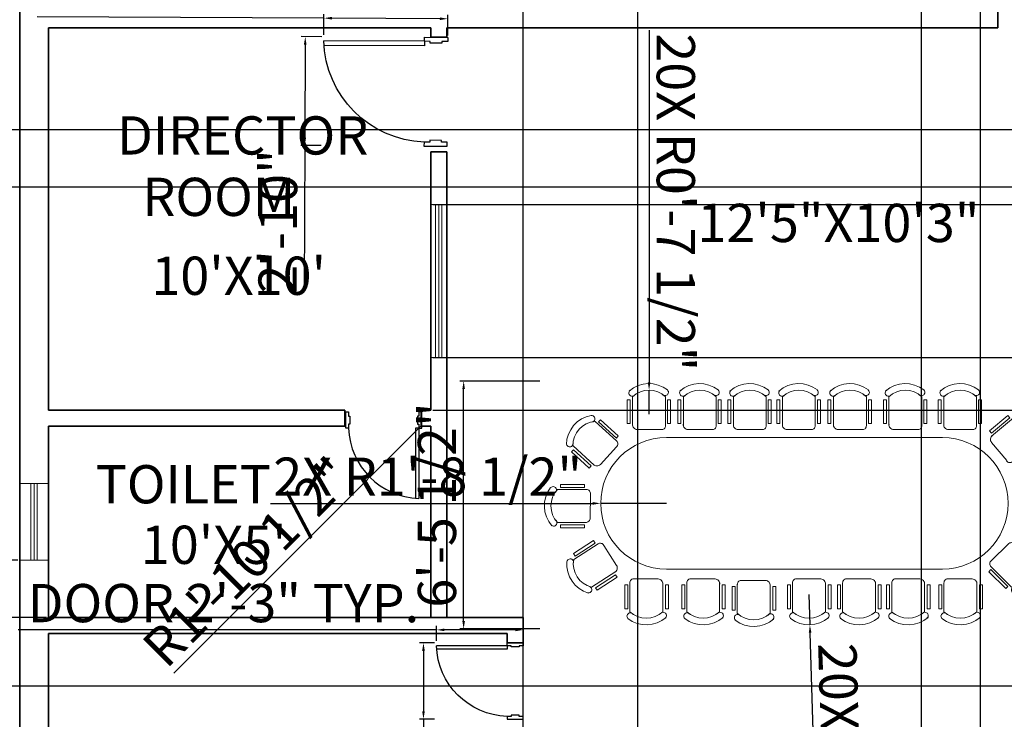
# Model space of a CAD drawing. Units: inches. Extents: x 2319 to 3765, y 2872 to 3950.
# Tile 3 of 9: x 2474 to 2783, y 3087 to 3306. Entities that reach past the tile are written whole.
import ezdxf

# ---------------------------------------------------------------- set-up
doc = ezdxf.new("R2010")
doc.units = ezdxf.units.IN
for name, color, linetype, lineweight in [('A-ANNO-DIMS', 2, 'Continuous', 18), ('A-ANNO-SYMB', 3, 'Continuous', 25), ('A-AREA-IDEN', 7, 'Continuous', 18), ('A-DOOR', 3, 'Continuous', 25), ('A-FURN', 8, 'Continuous', 18), ('A-GLAZ', 4, 'Continuous', 18), ('A-WALL', 7, 'Continuous', 35)]:
    doc.layers.add(name, color=color, linetype=linetype, lineweight=lineweight)
doc.styles.get("Standard").update_dxf_attribs({"font": 'arial.ttf'})
doc.dimstyles.new('ISO-25', dxfattribs={"dimtxt": 12, "dimasz": 2.5, "dimexe": 1.25, "dimexo": 0.625, "dimtad": 1, "dimdec": 0, "dimlunit": 3, "dimtxsty": 'Standard', "dimcen": 2.5, "dimadec": 0, "dimazin": 0, "dimtfac": 1, "dimtdec": 0, "dimtmove": 0, "dimatfit": 3, "dimfxl": 1, "dimarcsym": 0})

# ---------------------------------------------------------------- blocks, each defined once
blk = doc.blocks.new('A$C769D55ED')
for p, q in [((33.6, 192), (33.6, 1024.8)), ((72, 192), (72, 1023.9)), ((0, 192), (0, 0)), ((33.6, 192), (0, 192)), ((33.6, 144), (33.6, 192)), ((48, 144), (33.6, 144)), ((48, 48), (48, 144)), ((33.6, 0), (33.6, 48)), ((33.6, 48), (48, 48)), ((0, 0), (33.6, 0))]:
    blk.add_line(p, q)
blk.add_lwpolyline([(33.6, 192), (72, 192)])
blk.add_lwpolyline([(900, 192), (900, 0), (866.4, 0), (866.4, 48), (852, 48), (852, 144), (866.4, 144), (866.4, 192)], close=True)
blk.add_arc((7.2, 165.6), 859.6, 1.76235, 88.23765)
blk = doc.blocks.new('A$C0EDB4AB9')
at = {"linetype": 'ByBlock'}
for p, q in [((1257, 3447), (1257, 3084)), ((1303, 3447), (1257, 3447)), ((1303, 3084), (1303, 3447)), ((1342, 3055), (1342, 3493)), ((1842, 3493), (1842, 3051)), ((1873, 3447), (1873, 3084)), ((1919, 3447), (1873, 3447)), ((1919, 3084), (1919, 3447)), ((2028, 3447), (2028, 3084)), ((2074, 3447), (2028, 3447)), ((2074, 3084), (2074, 3447)), ((2114, 3055), (2114, 3493)), ((2614, 3493), (2614, 3051)), ((2644, 3447), (2644, 3084)), ((2691, 3447), (2644, 3447)), ((2691, 3084), (2691, 3447)), ((2790, 3447), (2790, 3084)), ((2836, 3447), (2790, 3447)), ((2836, 3084), (2836, 3447)), ((2875, 3055), (2875, 3493)), ((3375, 3493), (3375, 3051)), ((3406, 3447), (3406, 3084)), ((3452, 3447), (3406, 3447)), ((3452, 3084), (3452, 3447)), ((3537, 3447), (3537, 3084)), ((3583, 3447), (3537, 3447)), ((3583, 3084), (3583, 3447)), ((3622, 3055), (3622, 3493)), ((4122, 3493), (4122, 3051)), ((4153, 3447), (4153, 3084)), ((4199, 3447), (4153, 3447)), ((4199, 3084), (4199, 3447)), ((4314, 3447), (4314, 3084)), ((4360, 3447), (4314, 3447)), ((4360, 3084), (4360, 3447)), ((4399, 3055), (4399, 3493)), ((4899, 3493), (4899, 3051)), ((4930, 3447), (4930, 3084)), ((4976, 3447), (4930, 3447)), ((4976, 3084), (4976, 3447)), ((5158, 3447), (5158, 3084)), ((5204, 3447), (5158, 3447)), ((5204, 3084), (5204, 3447)), ((5243, 3055), (5243, 3493)), ((5743, 3493), (5743, 3051)), ((5774, 3447), (5774, 3084)), ((5820, 3447), (5774, 3447)), ((5820, 3084), (5820, 3447)), ((5991, 3447), (5991, 3084)), ((6037, 3447), (5991, 3447)), ((6037, 3084), (6037, 3447)), ((6076, 3055), (6076, 3493)), ((6576, 3493), (6576, 3051)), ((6607, 3447), (6607, 3084)), ((6653, 3447), (6607, 3447)), ((6653, 3084), (6653, 3447)), ((7050, 3209), (6772, 2975)), ((6802, 2940), (7080, 3173)), ((6804, 2891), (7139, 3172)), ((7080, 3173), (7050, 3209)), ((770, 3117), (1098, 2820)), ((855, 3143), (824, 3109)), ((824, 3109), (1094, 2865)), ((1124, 2900), (855, 3143)), ((1257, 3084), (1303, 3084)), ((1873, 3084), (1919, 3084)), ((2028, 3084), (2074, 3084)), ((2644, 3084), (2691, 3084)), ((2790, 3084), (2836, 3084)), ((3406, 3084), (3452, 3084)), ((3537, 3084), (3583, 3084)), ((4153, 3084), (4199, 3084)), ((4314, 3084), (4360, 3084)), ((4930, 3084), (4976, 3084)), ((5158, 3084), (5204, 3084)), ((5774, 3084), (5820, 3084)), ((5991, 3084), (6037, 3084)), ((6607, 3084), (6653, 3084)), ((1094, 2865), (1124, 2900)), ((1772, 2993), (1413, 2995)), ((1791, 2993), (1772, 2993)), ((6056, 2871), (1856, 2871)), ((2544, 2993), (2185, 2995)), ((2562, 2993), (2544, 2993)), ((3305, 2993), (2946, 2995)), ((3324, 2993), (3305, 2993)), ((4052, 2993), (3693, 2995)), ((4070, 2993), (4052, 2993)), ((4829, 2993), (4470, 2995)), ((4847, 2993), (4829, 2993)), ((5673, 2993), (5314, 2995)), ((5692, 2993), (5673, 2993)), ((6506, 2993), (6147, 2995)), ((6525, 2993), (6506, 2993)), ((6772, 2975), (6802, 2940)), ((759, 2452), (435, 2746)), ((1094, 2729), (851, 2464)), ((1106, 2743), (1094, 2729)), ((7034, 2521), (6804, 2798)), ((7461, 2790), (7123, 2505)), ((7446, 2737), (7169, 2503)), ((7198, 2468), (7476, 2702)), ((7476, 2702), (7446, 2737)), ((442, 2687), (411, 2653)), ((411, 2653), (680, 2409)), ((711, 2443), (442, 2687)), ((680, 2409), (711, 2443)), ((7169, 2503), (7198, 2468)), ((608, 2159), (245, 2159)), ((245, 2159), (245, 2113)), ((245, 2113), (608, 2113)), ((608, 2113), (608, 2159)), ((7227, 2127), (7665, 2127)), ((7619, 2213), (7256, 2213)), ((7256, 2213), (7256, 2167)), ((7256, 2167), (7619, 2167)), ((7619, 2167), (7619, 2213)), ((200, 2082), (642, 2082)), ((700, 2012), (698, 1653)), ((700, 2031), (700, 2012)), ((7165, 1697), (7167, 2056)), ((7165, 1679), (7165, 1697)), ((638, 1582), (200, 1582)), ((608, 1543), (245, 1543)), ((245, 1543), (245, 1497)), ((608, 1497), (608, 1543)), ((7665, 1627), (7223, 1627)), ((7619, 1597), (7256, 1597)), ((7256, 1597), (7256, 1550)), ((7256, 1550), (7619, 1550)), ((7619, 1550), (7619, 1597)), ((245, 1497), (608, 1497)), ((748, 1304), (442, 1107)), ((446, 1018), (817, 1257)), ((467, 1068), (772, 1265)), ((772, 1265), (748, 1304)), ((894, 1245), (904, 1230)), ((904, 1230), (1097, 927)), ((6802, 1000), (7057, 1253)), ((7150, 1260), (7459, 951)), ((7231, 1300), (7198, 1267)), ((7198, 1267), (7455, 1011)), ((7487, 1043), (7231, 1300)), ((442, 1107), (467, 1068)), ((6788, 987), (6802, 1000)), ((7106, 597), (6793, 909)), ((7455, 1011), (7487, 1043)), ((1084, 834), (716, 598)), ((1081, 786), (776, 589)), ((1106, 747), (1081, 786)), ((6056, 871), (1856, 871)), ((6795, 864), (6763, 831)), ((6763, 831), (7019, 575)), ((7052, 607), (6795, 864)), ((800, 550), (1106, 747)), ((1270, 632), (1224, 632)), ((1224, 632), (1224, 269)), ((1270, 269), (1270, 632)), ((1300, 223), (1300, 665)), ((1352, 723), (1370, 723)), ((1370, 723), (1730, 722)), ((1800, 661), (1800, 223)), ((1886, 632), (1840, 632)), ((1840, 632), (1840, 269)), ((1886, 269), (1886, 632)), ((2135, 632), (2089, 632)), ((2089, 632), (2089, 269)), ((2135, 269), (2135, 632)), ((2166, 223), (2166, 665)), ((2218, 723), (2236, 723)), ((2236, 723), (2595, 722)), ((2666, 661), (2666, 223)), ((2752, 632), (2705, 632)), ((2705, 632), (2705, 269)), ((2752, 269), (2752, 632)), ((2904, 608), (2858, 608)), ((2858, 608), (2858, 245)), ((2904, 245), (2904, 608)), ((2935, 200), (2935, 642)), ((2986, 700), (3005, 700)), ((3005, 700), (3364, 698)), ((3435, 638), (3435, 200)), ((3520, 608), (3474, 608)), ((3474, 608), (3474, 245)), ((3520, 245), (3520, 608)), ((3745, 632), (3699, 632)), ((3699, 632), (3699, 269)), ((3745, 269), (3745, 632)), ((3776, 223), (3776, 665)), ((3827, 723), (3846, 723)), ((3846, 723), (4205, 722)), ((4276, 661), (4276, 223)), ((4361, 632), (4315, 632)), ((4315, 632), (4315, 269)), ((4361, 269), (4361, 632)), ((4507, 632), (4461, 632)), ((4461, 632), (4461, 269)), ((4507, 269), (4507, 632)), ((4537, 223), (4537, 665)), ((4589, 723), (4607, 723)), ((4607, 723), (4966, 722)), ((5037, 661), (5037, 223)), ((5123, 632), (5077, 632)), ((5077, 632), (5077, 269)), ((5123, 269), (5123, 632)), ((5253, 632), (5207, 632)), ((5207, 632), (5207, 269)), ((5253, 269), (5253, 632)), ((5284, 223), (5284, 665)), ((5335, 723), (5354, 723)), ((5354, 723), (5713, 722)), ((5784, 661), (5784, 223)), ((5869, 632), (5823, 632)), ((5823, 632), (5823, 269)), ((5869, 269), (5869, 632)), ((6049, 632), (6003, 632)), ((6003, 632), (6003, 269)), ((6049, 269), (6049, 632)), ((6079, 223), (6079, 665)), ((6131, 723), (6149, 723)), ((6149, 723), (6508, 722)), ((6579, 661), (6579, 223)), ((6665, 632), (6619, 632)), ((6619, 632), (6619, 269)), ((6665, 269), (6665, 632)), ((7019, 575), (7052, 607)), ((776, 589), (800, 550)), ((1224, 269), (1270, 269)), ((1840, 269), (1886, 269)), ((2089, 269), (2135, 269)), ((2705, 269), (2752, 269)), ((2858, 245), (2904, 245)), ((3474, 245), (3520, 245)), ((3699, 269), (3745, 269)), ((4315, 269), (4361, 269)), ((4461, 269), (4507, 269)), ((5077, 269), (5123, 269)), ((5207, 269), (5253, 269)), ((5823, 269), (5869, 269)), ((6003, 269), (6049, 269)), ((6619, 269), (6665, 269))]:
    blk.add_line(p, q, dxfattribs=at)
for centre, radius, start, end in [((1592, 3230), 463, 52.6032, 130.8409), ((1837, 3560), 50, 219.1941, 46.1701), ((2364, 3230), 463, 52.6032, 130.8409), ((2609, 3560), 50, 219.1941, 46.1701), ((3125, 3230), 463, 52.6032, 130.8409), ((3370, 3560), 50, 219.1941, 46.1701), ((3872, 3230), 463, 52.6032, 130.8409), ((4117, 3560), 50, 219.1941, 46.1701), ((4649, 3230), 463, 52.6032, 130.8409), ((4894, 3560), 50, 219.1941, 46.1701), ((5493, 3230), 463, 52.6032, 130.8409), ((5738, 3560), 50, 219.1941, 46.1701), ((6326, 3230), 463, 52.6032, 130.8409), ((6571, 3560), 50, 219.1941, 46.1701), ((1335, 3551), 50, 127.3845, 320.4832), ((1592, 3230), 363, 46.3972, 133.6028), ((2107, 3551), 50, 127.3845, 320.4832), ((2364, 3230), 363, 46.3972, 133.6028), ((2869, 3551), 50, 127.3845, 320.4832), ((3125, 3230), 363, 46.3972, 133.6028), ((3615, 3551), 50, 127.3845, 320.4832), ((3872, 3230), 363, 46.3972, 133.6028), ((4392, 3551), 50, 127.3845, 320.4832), ((4649, 3230), 363, 46.3972, 133.6028), ((5236, 3551), 50, 127.3845, 320.4832), ((5493, 3230), 363, 46.3972, 133.6028), ((6069, 3551), 50, 127.3845, 320.4832), ((6326, 3230), 363, 46.3972, 133.6028), ((797, 2755), 463, 100.4356, 178.6733), ((717, 3158), 50, 267.0265, 94.0025), ((7180, 3215), 50, 77.4483, 270.5471), ((7100, 2812), 363, 356.461, 83.6667), ((7100, 2812), 463, 2.6671, 80.9047), ((797, 2755), 363, 94.2296, 181.4352), ((1412, 3065), 70.2, 172.0281, 271.1673), ((1782, 3053), 60.7, 261.2421, 1.6502), ((2183, 3065), 70.2, 172.0281, 271.1673), ((2553, 3053), 60.7, 261.2421, 1.6502), ((2945, 3065), 70.2, 172.0281, 271.1673), ((3315, 3053), 60.7, 261.2421, 1.6502), ((3691, 3065), 70.2, 172.0281, 271.1673), ((4061, 3053), 60.7, 261.2421, 1.6502), ((4468, 3065), 70.2, 172.0281, 271.1673), ((4838, 3053), 60.7, 261.2421, 1.6502), ((5313, 3065), 70.2, 172.0281, 271.1673), ((5682, 3053), 60.7, 261.2421, 1.6502), ((6146, 3065), 70.2, 172.0281, 271.1673), ((6515, 3053), 60.7, 261.2421, 1.6502), ((1856, 1871), 1000, 90, 270), ((6056, 1871), 1000, 270, 90), ((6857, 2844), 70.2, 122.0919, 221.2312), ((386, 2780), 50, 175.2169, 8.3156), ((1056, 2776), 60.7, 309.0745, 49.4826), ((7510, 2837), 50, 169.258, 356.234), ((798, 2510), 70.2, 219.8605, 318.9997), ((7083, 2551), 60.7, 211.3059, 311.714), ((462, 1832), 463, 142.6032, 220.8409), ((132, 2077), 50, 309.1941, 136.1701), ((7237, 2058), 70.2, 82.0281, 181.1673), ((7402, 1877), 363, 316.3972, 43.6028), ((7723, 2134), 50, 37.3845, 230.4832), ((7402, 1877), 463, 322.6032, 40.8409), ((462, 1832), 363, 136.3972, 223.6028), ((640, 2021), 60.7, 351.2421, 91.6502), ((628, 1651), 70.2, 262.0281, 1.1673), ((7225, 1688), 60.7, 171.2421, 271.6502), ((7732, 1632), 50, 129.1941, 316.1701), ((141, 1575), 50, 217.3845, 50.4832), ((848, 1205), 60.7, 24.0035, 124.4116), ((7107, 1204), 70.2, 37.0567, 136.1959), ((802, 950), 463, 175.3647, 253.6023), ((392, 977), 50, 341.9556, 168.9315), ((802, 950), 363, 169.1586, 256.3643), ((1039, 888), 70.2, 294.7895, 33.9288), ((6837, 951), 60.7, 126.2707, 226.6788), ((7097, 960), 363, 271.4258, 358.6314), ((7097, 960), 463, 277.6319, 355.8695), ((7506, 914), 50, 352.4131, 185.5118), ((671, 560), 50, 250.1459, 83.2447), ((1361, 663), 60.7, 81.2421, 181.6502), ((1731, 651), 70.2, 352.0281, 91.1673), ((2227, 663), 60.7, 81.2421, 181.6502), ((2597, 651), 70.2, 352.0281, 91.1673), ((2996, 640), 60.7, 81.2421, 181.6502), ((3365, 628), 70.2, 352.0281, 91.1673), ((3836, 663), 60.7, 81.2421, 181.6502), ((4206, 651), 70.2, 352.0281, 91.1673), ((4598, 663), 60.7, 81.2421, 181.6502), ((4968, 651), 70.2, 352.0281, 91.1673), ((5345, 663), 60.7, 81.2421, 181.6502), ((5714, 651), 70.2, 352.0281, 91.1673), ((6140, 663), 60.7, 81.2421, 181.6502), ((6510, 651), 70.2, 352.0281, 91.1673), ((7157, 553), 50, 84.2228, 271.1987), ((1306, 156), 50, 39.1941, 226.1701), ((1550, 486), 363, 226.3972, 313.6028), ((1807, 165), 50, 307.3845, 140.4832), ((2171, 156), 50, 39.1941, 226.1701), ((2416, 486), 363, 226.3972, 313.6028), ((2673, 165), 50, 307.3845, 140.4832), ((2940, 132), 50, 39.1941, 226.1701), ((3185, 462), 363, 226.3972, 313.6028), ((3442, 141), 50, 307.3845, 140.4832), ((3781, 156), 50, 39.1941, 226.1701), ((4026, 486), 363, 226.3972, 313.6028), ((4283, 165), 50, 307.3845, 140.4832), ((4543, 156), 50, 39.1941, 226.1701), ((4787, 486), 363, 226.3972, 313.6028), ((5044, 165), 50, 307.3845, 140.4832), ((5289, 156), 50, 39.1941, 226.1701), ((5534, 486), 363, 226.3972, 313.6028), ((5791, 165), 50, 307.3845, 140.4832), ((6084, 156), 50, 39.1941, 226.1701), ((6329, 486), 363, 226.3972, 313.6028), ((6586, 165), 50, 307.3845, 140.4832), ((1550, 486), 463, 232.6032, 310.8409), ((2416, 486), 463, 232.6032, 310.8409), ((3185, 462), 463, 232.6032, 310.8409), ((4026, 486), 463, 232.6032, 310.8409), ((4787, 486), 463, 232.6032, 310.8409), ((5534, 486), 463, 232.6032, 310.8409), ((6329, 486), 463, 232.6032, 310.8409)]:
    blk.add_arc(centre, radius, start, end, dxfattribs=at)
blk = doc.blocks.new('*D53')
at = {"layer": 'A-ANNO-DIMS', "color": 0, "lineweight": -2, "transparency": 16777216}
for p, q in [((2604.93, 3111.24), (2604.93, 3115.95)), ((2632.18, 3111.24), (2632.18, 3115.95)), ((2604.93, 3114.7), (2473.68, 3114.7)), ((2629.68, 3114.7), (2607.43, 3114.7))]:
    blk.add_line(p, q, dxfattribs=at)
at = {"layer": 'A-ANNO-DIMS', "color": 0, "transparency": 16777216}
for points in [[(2607.43, 3115.11), (2607.43, 3114.28), (2604.93, 3114.7)], [(2629.68, 3115.11), (2629.68, 3114.28), (2632.18, 3114.7)]]:
    blk.add_solid(points, dxfattribs=at)
at = {"layer": 'Defpoints', "color": 0, "transparency": 16777216}
for p in [(2604.93, 3114.7), (2604.93, 3110.61), (2632.18, 3110.61)]:
    blk.add_point(p, dxfattribs=at)
at = {"layer": 'A-ANNO-DIMS', "color": 0, "transparency": 16777216, "insert": (2538.06, 3121.54), "char_height": 12, "attachment_point": 5}
blk.add_mtext('DOOR 2\'-3" TYP.', dxfattribs=at)
blk = doc.blocks.new('*D54')
at = {"layer": 'A-ANNO-DIMS', "color": 0, "lineweight": -2, "transparency": 16777216}
for p, q in [((2604.31, 3110.61), (2599.6, 3110.61)), ((2600.85, 3108.11), (2600.85, 3089.18)), ((2604.31, 3086.68), (2599.6, 3086.68)), ((2600.85, 3086.68), (2600.85, 3009.58))]:
    blk.add_line(p, q, dxfattribs=at)
at = {"layer": 'A-ANNO-DIMS', "color": 0, "transparency": 16777216}
for points in [[(2600.43, 3108.11), (2601.26, 3108.11), (2600.85, 3110.61)], [(2600.43, 3089.18), (2601.26, 3089.18), (2600.85, 3086.68)]]:
    blk.add_solid(points, dxfattribs=at)
at = {"layer": 'Defpoints', "color": 0, "transparency": 16777216}
for p in [(2604.93, 3110.61), (2600.85, 3086.68), (2604.93, 3086.68)]:
    blk.add_point(p, dxfattribs=at)
at = {"layer": 'A-ANNO-DIMS', "color": 0, "transparency": 16777216, "insert": (2594.09, 3046.88), "char_height": 12, "attachment_point": 5, "rotation": 90}
blk.add_mtext('2\'-0" TYP.', dxfattribs=at)
blk = doc.blocks.new('*D55')
at = {"layer": 'A-ANNO-DIMS', "color": 0, "lineweight": -2, "transparency": 16777216}
for p, q in [((2569.61, 3306.59), (2479.61, 3307.04)), ((2569.58, 3301.38), (2569.62, 3307.84)), ((2605.99, 3306.41), (2572.11, 3306.58)), ((2608.46, 3301.19), (2608.49, 3307.65))]:
    blk.add_line(p, q, dxfattribs=at)
at = {"layer": 'A-ANNO-DIMS', "color": 0, "transparency": 16777216}
for points in [[(2572.11, 3307), (2572.11, 3306.16), (2569.61, 3306.59)], [(2605.99, 3306.83), (2605.98, 3305.99), (2608.49, 3306.4)]]:
    blk.add_solid(points, dxfattribs=at)
at = {"layer": 'Defpoints', "color": 0, "transparency": 16777216}
for p in [(2569.61, 3306.59), (2569.58, 3300.76), (2608.46, 3300.57)]:
    blk.add_point(p, dxfattribs=at)
at = {"layer": 'A-ANNO-DIMS', "color": 0, "transparency": 16777216, "insert": (2523.39, 3313.66), "char_height": 12, "attachment_point": 5, "rotation": 359.7171}
blk.add_mtext('DOOR 3\'-3"', dxfattribs=at)
blk = doc.blocks.new('*D56')
at = {"layer": 'A-ANNO-DIMS', "color": 0, "lineweight": -2, "transparency": 16777216}
for p, q in [((2568.96, 3300.76), (2562.5, 3300.79)), ((2563.74, 3298.29), (2563.59, 3269.15)), ((2568.79, 3266.62), (2562.33, 3266.65)), ((2563.58, 3266.65), (2563.36, 3221.47))]:
    blk.add_line(p, q, dxfattribs=at)
at = {"layer": 'A-ANNO-DIMS', "color": 0, "transparency": 16777216}
for points in [[(2563.32, 3298.29), (2564.15, 3298.29), (2563.75, 3300.79)], [(2563.18, 3269.15), (2564.01, 3269.14), (2563.58, 3266.65)]]:
    blk.add_solid(points, dxfattribs=at)
at = {"layer": 'Defpoints', "color": 0, "transparency": 16777216}
for p in [(2569.58, 3300.76), (2563.58, 3266.65), (2569.41, 3266.62)]:
    blk.add_point(p, dxfattribs=at)
at = {"layer": 'A-ANNO-DIMS', "color": 0, "transparency": 16777216, "insert": (2556.71, 3242.84), "char_height": 12, "attachment_point": 5, "rotation": 89.7171}
blk.add_mtext('2\'-10"', dxfattribs=at)
blk = doc.blocks.new('*D64')
at = {"layer": 'A-ANNO-DIMS', "color": 0, "lineweight": -2, "transparency": 16777216}
for p, q in [((2637.4, 3192.74), (2612.21, 3192.74)), ((2613.46, 3117.51), (2613.46, 3190.24)), ((2637.4, 3115.01), (2612.21, 3115.01))]:
    blk.add_line(p, q, dxfattribs=at)
at = {"layer": 'A-ANNO-DIMS', "color": 0, "transparency": 16777216}
for points in [[(2613.04, 3190.24), (2613.87, 3190.24), (2613.46, 3192.74)], [(2613.04, 3117.51), (2613.87, 3117.51), (2613.46, 3115.01)]]:
    blk.add_solid(points, dxfattribs=at)
at = {"layer": 'Defpoints', "color": 0, "transparency": 16777216}
for p in [(2613.46, 3192.74), (2638.02, 3192.74), (2638.02, 3115.01)]:
    blk.add_point(p, dxfattribs=at)
at = {"layer": 'A-ANNO-DIMS', "color": 0, "transparency": 16777216, "insert": (2606.63, 3153.87), "char_height": 12, "attachment_point": 5, "rotation": 90}
blk.add_mtext('6\'-5 1/2"', dxfattribs=at)
blk = doc.blocks.new('*D75')
at = {"layer": 'A-ANNO-DIMS', "color": 0, "lineweight": -2, "transparency": 16777216}
for p, q in [((2632.13, 2970.24), (2632.13, 3605.01)), ((2634.63, 3603.76), (2665.63, 3603.76)), ((2668.13, 2970.24), (2668.13, 3605.01))]:
    blk.add_line(p, q, dxfattribs=at)
at = {"layer": 'A-ANNO-DIMS', "color": 0, "transparency": 16777216}
for points in [[(2634.63, 3604.18), (2634.63, 3603.34), (2632.13, 3603.76)], [(2665.63, 3604.18), (2665.63, 3603.34), (2668.13, 3603.76)]]:
    blk.add_solid(points, dxfattribs=at)
at = {"layer": 'Defpoints', "color": 0, "transparency": 16777216}
for p in [(2668.13, 3603.76), (2632.13, 2969.61), (2668.13, 2969.61)]:
    blk.add_point(p, dxfattribs=at)
at = {"layer": 'A-ANNO-DIMS', "color": 0, "transparency": 16777216, "insert": (2650.13, 3610.52), "char_height": 12, "attachment_point": 5}
blk.add_mtext('3\'-0"', dxfattribs=at)
blk = doc.blocks.new('*D76')
at = {"layer": 'A-ANNO-DIMS', "color": 0, "lineweight": -2, "transparency": 16777216}
for p, q in [((2757.13, 2970.24), (2757.13, 3605.01)), ((2759.63, 3603.76), (2773.17, 3603.76)), ((2775.67, 2970.24), (2775.67, 3605.01)), ((2775.67, 3603.76), (2838.15, 3603.76))]:
    blk.add_line(p, q, dxfattribs=at)
at = {"layer": 'A-ANNO-DIMS', "color": 0, "transparency": 16777216}
for points in [[(2759.63, 3604.18), (2759.63, 3603.34), (2757.13, 3603.76)], [(2773.17, 3604.18), (2773.17, 3603.34), (2775.67, 3603.76)]]:
    blk.add_solid(points, dxfattribs=at)
at = {"layer": 'Defpoints', "color": 0, "transparency": 16777216}
for p in [(2775.67, 3603.76), (2757.13, 2969.61), (2775.67, 2969.61)]:
    blk.add_point(p, dxfattribs=at)
at = {"layer": 'A-ANNO-DIMS', "color": 0, "transparency": 16777216, "insert": (2808.16, 3610.59), "char_height": 12, "attachment_point": 5}
blk.add_mtext('1\'-6 1/2"', dxfattribs=at)
blk = doc.blocks.new('*D80')
at = {"layer": 'A-ANNO-DIMS', "color": 0, "lineweight": -2, "transparency": 16777216}
for p, q in [((2343.14, 3136.61), (2343.14, 3171.13)), ((2473.5, 3136.61), (2341.89, 3136.61)), ((2343.14, 3121.11), (2343.14, 3134.11)), ((2482.5, 3118.61), (2341.89, 3118.61))]:
    blk.add_line(p, q, dxfattribs=at)
at = {"layer": 'A-ANNO-DIMS', "color": 0, "transparency": 16777216}
for points in [[(2342.72, 3134.11), (2343.56, 3134.11), (2343.14, 3136.61)], [(2342.72, 3121.11), (2343.56, 3121.11), (2343.14, 3118.61)]]:
    blk.add_solid(points, dxfattribs=at)
at = {"layer": 'Defpoints', "color": 0, "transparency": 16777216}
for p in [(2343.14, 3136.61), (2474.13, 3136.61), (2483.13, 3118.61)]:
    blk.add_point(p, dxfattribs=at)
at = {"layer": 'A-ANNO-DIMS', "color": 0, "transparency": 16777216, "insert": (2336.39, 3155.12), "char_height": 12, "attachment_point": 5, "rotation": 90}
blk.add_mtext('1\'-6"', dxfattribs=at)
blk = doc.blocks.new('*D81')
at = {"layer": 'A-ANNO-DIMS', "color": 0, "lineweight": -2, "transparency": 16777216}
for p, q in [((2603.75, 3248.11), (3085.2, 3248.11)), ((3083.95, 3202.61), (3083.95, 3245.61)), ((2603.75, 3200.11), (3085.2, 3200.11))]:
    blk.add_line(p, q, dxfattribs=at)
at = {"layer": 'A-ANNO-DIMS', "color": 0, "transparency": 16777216}
for points in [[(3083.53, 3245.61), (3084.36, 3245.61), (3083.95, 3248.11)], [(3083.53, 3202.61), (3084.36, 3202.61), (3083.95, 3200.11)]]:
    blk.add_solid(points, dxfattribs=at)
at = {"layer": 'Defpoints', "color": 0, "transparency": 16777216}
for p in [(2603.13, 3248.11), (3083.95, 3248.11), (2603.13, 3200.11)]:
    blk.add_point(p, dxfattribs=at)
at = {"layer": 'A-ANNO-DIMS', "color": 0, "transparency": 16777216, "insert": (3077.2, 3224.11), "char_height": 12, "attachment_point": 5, "rotation": 90}
blk.add_mtext('4\'-0"', dxfattribs=at)
blk = doc.blocks.new('*D82')
at = {"layer": 'A-ANNO-DIMS', "color": 0, "lineweight": -2, "transparency": 16777216}
for p, q in [((3083.95, 3200.11), (3083.95, 3262.59)), ((2603.75, 3200.11), (3085.2, 3200.11)), ((3083.95, 3186.11), (3083.95, 3197.61)), ((2603.75, 3183.61), (3085.2, 3183.61))]:
    blk.add_line(p, q, dxfattribs=at)
at = {"layer": 'A-ANNO-DIMS', "color": 0, "transparency": 16777216}
for points in [[(3083.53, 3197.61), (3084.36, 3197.61), (3083.95, 3200.11)], [(3083.53, 3186.11), (3084.36, 3186.11), (3083.95, 3183.61)]]:
    blk.add_solid(points, dxfattribs=at)
at = {"layer": 'Defpoints', "color": 0, "transparency": 16777216}
for p in [(2603.13, 3200.11), (3083.95, 3200.11), (2603.13, 3183.61)]:
    blk.add_point(p, dxfattribs=at)
at = {"layer": 'A-ANNO-DIMS', "color": 0, "transparency": 16777216, "insert": (3077.12, 3232.6), "char_height": 12, "attachment_point": 5, "rotation": 90}
blk.add_mtext('1\'-4 1/2"', dxfattribs=at)
blk = doc.blocks.new('*D87')
at = {"layer": 'A-ANNO-DIMS', "color": 0, "lineweight": -2, "transparency": 16777216}
for p, q in [((2800.5, 3380.11), (2341.89, 3380.11)), ((2343.14, 3377.61), (2343.14, 3360.11)), ((2800.5, 3357.61), (2341.89, 3357.61)), ((2343.14, 3357.61), (2343.14, 3285.81))]:
    blk.add_line(p, q, dxfattribs=at)
at = {"layer": 'A-ANNO-DIMS', "color": 0, "transparency": 16777216}
for points in [[(2342.72, 3377.61), (2343.56, 3377.61), (2343.14, 3380.11)], [(2342.72, 3360.11), (2343.56, 3360.11), (2343.14, 3357.61)]]:
    blk.add_solid(points, dxfattribs=at)
at = {"layer": 'Defpoints', "color": 0, "transparency": 16777216}
for p in [(2801.13, 3380.11), (2343.14, 3357.61), (2801.13, 3357.61)]:
    blk.add_point(p, dxfattribs=at)
at = {"layer": 'A-ANNO-DIMS', "color": 0, "transparency": 16777216, "insert": (2336.31, 3320.46), "char_height": 12, "attachment_point": 5, "rotation": 90}
blk.add_mtext('1\'-10 1/2"', dxfattribs=at)
blk = doc.blocks.new('*D88')
at = {"layer": 'A-ANNO-DIMS', "color": 0, "lineweight": -2, "transparency": 16777216}
for p, q in [((2343.14, 3271.61), (2343.14, 3306.13)), ((2949.5, 3271.61), (2341.89, 3271.61)), ((2343.14, 3256.11), (2343.14, 3269.11)), ((2949.5, 3253.61), (2341.89, 3253.61))]:
    blk.add_line(p, q, dxfattribs=at)
at = {"layer": 'A-ANNO-DIMS', "color": 0, "transparency": 16777216}
for points in [[(2342.72, 3269.11), (2343.56, 3269.11), (2343.14, 3271.61)], [(2342.72, 3256.11), (2343.56, 3256.11), (2343.14, 3253.61)]]:
    blk.add_solid(points, dxfattribs=at)
at = {"layer": 'Defpoints', "color": 0, "transparency": 16777216}
for p in [(2343.14, 3271.61), (2950.13, 3271.61), (2950.13, 3253.61)]:
    blk.add_point(p, dxfattribs=at)
at = {"layer": 'A-ANNO-DIMS', "color": 0, "transparency": 16777216, "insert": (2336.39, 3290.12), "char_height": 12, "attachment_point": 5, "rotation": 90}
blk.add_mtext('1\'-6"', dxfattribs=at)
blk = doc.blocks.new('*D104')
at = {"layer": 'A-ANNO-DIMS', "color": 0, "lineweight": -2, "transparency": 16777216}
for p, q in [((2600.09, 3178.68), (2584.01, 3162.61)), ((2522.55, 3101.15), (2582.25, 3160.84))]:
    blk.add_line(p, q, dxfattribs=at)
at = {"layer": 'A-ANNO-DIMS', "color": 0, "transparency": 16777216}
blk.add_solid([(2581.95, 3161.13), (2582.54, 3160.54), (2584.01, 3162.61)], dxfattribs=at)
at = {"layer": 'Defpoints', "color": 0, "transparency": 16777216}
for p in [(2600.09, 3178.68), (2584.01, 3162.61)]:
    blk.add_point(p, dxfattribs=at)
at = {"layer": 'A-ANNO-DIMS', "color": 0, "transparency": 16777216, "insert": (2546.69, 3134.94), "char_height": 12, "attachment_point": 5, "rotation": 44.9997}
blk.add_mtext('R1\'-10 1/2"', dxfattribs=at)
blk = doc.blocks.new('*D105')
at = {"layer": 'A-ANNO-DIMS', "color": 0, "lineweight": -2, "transparency": 16777216}
for p, q in [((2552.88, 3154.38), (2653.96, 3154.38)), ((2677.09, 3154.38), (2656.46, 3154.38))]:
    blk.add_line(p, q, dxfattribs=at)
at = {"layer": 'A-ANNO-DIMS', "color": 0, "transparency": 16777216}
blk.add_solid([(2653.96, 3154.79), (2653.96, 3153.96), (2656.46, 3154.38)], dxfattribs=at)
at = {"layer": 'Defpoints', "color": 0, "transparency": 16777216}
for p in [(2656.46, 3154.38), (2677.09, 3154.38)]:
    blk.add_point(p, dxfattribs=at)
at = {"layer": 'A-ANNO-DIMS', "color": 0, "transparency": 16777216, "insert": (2602.17, 3161.21), "char_height": 12, "attachment_point": 5, "rotation": 0.0006}
blk.add_mtext('2X R1\'-8 1/2"', dxfattribs=at)
blk = doc.blocks.new('*D106')
at = {"layer": 'A-ANNO-DIMS', "color": 0, "lineweight": -2, "transparency": 16777216}
for p, q in [((2721.83, 3125.82), (2722.12, 3116.28)), ((2725.52, 3003.42), (2722.2, 3113.78))]:
    blk.add_line(p, q, dxfattribs=at)
at = {"layer": 'A-ANNO-DIMS', "color": 0, "transparency": 16777216}
blk.add_solid([(2722.61, 3113.79), (2721.78, 3113.77), (2722.12, 3116.28)], dxfattribs=at)
at = {"layer": 'Defpoints', "color": 0, "transparency": 16777216}
for p in [(2721.83, 3125.82), (2722.12, 3116.28)]:
    blk.add_point(p, dxfattribs=at)
at = {"layer": 'A-ANNO-DIMS', "color": 0, "transparency": 16777216, "insert": (2730.72, 3057.56), "char_height": 12, "attachment_point": 5, "rotation": 271.7247}
blk.add_mtext('20X R0\'-9 1/2"', dxfattribs=at)
blk = doc.blocks.new('*D107')
at = {"layer": 'A-ANNO-DIMS', "color": 0, "lineweight": -2, "transparency": 16777216}
for p, q in [((2671.64, 3302.8), (2671.65, 3192.39)), ((2671.65, 3182.41), (2671.65, 3189.89))]:
    blk.add_line(p, q, dxfattribs=at)
at = {"layer": 'A-ANNO-DIMS', "color": 0, "transparency": 16777216}
blk.add_solid([(2672.07, 3192.39), (2671.23, 3192.39), (2671.65, 3189.89)], dxfattribs=at)
at = {"layer": 'Defpoints', "color": 0, "transparency": 16777216}
for p in [(2671.65, 3189.89), (2671.65, 3182.41)]:
    blk.add_point(p, dxfattribs=at)
at = {"layer": 'A-ANNO-DIMS', "color": 0, "transparency": 16777216, "insert": (2678.48, 3248.84), "char_height": 12, "attachment_point": 5, "rotation": 270.0036}
blk.add_mtext('20X R0\'-7 1/2"', dxfattribs=at)

msp = doc.modelspace()

# ---------------------------------------------------------------- linework, layer by layer
at = {"layer": 'A-ANNO-SYMB'}
msp.add_line((3034.33, 3097.01), (2389.37, 3097.01), dxfattribs=at)
at = {"layer": 'A-GLAZ'}
for p, q in [((2603.13, 3248.11), (2608.13, 3248.11)), ((2604.63, 3200.11), (2604.63, 3248.11)), ((2605.63, 3200.11), (2605.63, 3248.11)), ((2606.63, 3200.11), (2606.63, 3248.11)), ((2603.13, 3200.11), (2608.13, 3200.11)), ((2483.13, 3160.61), (2474.13, 3160.61)), ((2477.63, 3136.61), (2477.63, 3160.61)), ((2478.63, 3136.61), (2478.63, 3160.61)), ((2479.63, 3136.61), (2479.63, 3160.61)), ((2483.13, 3136.61), (2474.13, 3136.61))]:
    msp.add_line(p, q, dxfattribs=at)
at = {"layer": 'A-WALL'}
for p, q in [((2474.13, 2960.61), (2474.13, 3458.61)), ((2781.13, 3308.61), (2781.13, 3303.61)), ((2483.13, 3183.61), (2483.13, 3303.61)), ((2483.13, 3303.61), (2603.13, 3303.61)), ((2603.13, 3303.61), (2603.13, 3300.61)), ((2608.13, 3303.61), (2608.13, 3300.61)), ((2608.13, 3303.61), (2781.13, 3303.61)), ((2608.13, 3300.61), (2603.13, 3300.61)), ((2608.13, 3264.61), (2603.13, 3264.61)), ((2603.13, 3264.61), (2603.13, 3183.61)), ((2608.13, 3264.61), (2608.13, 3118.61)), ((2483.13, 3183.61), (2576.13, 3183.61)), ((2576.13, 3183.61), (2576.13, 3178.61)), ((2600.13, 3183.61), (2600.13, 3178.61)), ((2600.13, 3183.61), (2603.13, 3183.61)), ((2483.13, 3118.61), (2483.13, 3178.61)), ((2483.13, 3178.61), (2576.13, 3178.61)), ((2600.13, 3178.61), (2603.13, 3178.61)), ((2603.13, 3178.61), (2603.13, 3118.61)), ((2483.13, 3118.61), (2632.13, 3118.61)), ((2632.13, 3110.61), (2632.13, 3118.61)), ((2483.13, 3113.61), (2627.13, 3113.61)), ((2483.13, 2969.61), (2483.13, 3113.61)), ((2627.13, 3110.61), (2627.13, 3113.61)), ((2627.13, 3110.61), (2632.13, 3110.61))]:
    msp.add_line(p, q, dxfattribs=at)

# ---------------------------------------------------------------- block references
at = {"layer": 'A-DOOR'}
for p, xscale, yscale, zscale, rotation in [((2608.46, 3300.57), -0.0379354334797352, 0.0379354334797352, 0.0379354334797352, 89.717129223989), ((2600.28, 3183.06), 0.0264456636432611, 0.0264456636432611, 0.0264456636432611, 180), ((2632.18, 3110.61), -0.0265876055345398, 0.0265876055345398, 0.0265876055345398, 90)]:
    msp.add_blockref('A$C769D55ED', p, dxfattribs=dict(at, xscale=xscale, yscale=yscale, zscale=zscale, rotation=rotation))
at = {"layer": 'A-FURN', "xscale": 0.02062408179219, "yscale": 0.02062408179219, "zscale": 0.02062408179219}
msp.add_blockref('A$C0EDB4AB9', (2638.81, 3115.79), dxfattribs=at)

# ---------------------------------------------------------------- texts
at = {"layer": 'A-AREA-IDEN'}
for s, p in [('DIRECTOR ', (2504.66, 3263.81)), ('ROOM', (2512.61, 3244.53)), ('12\'5"X10\'3"', (2686.84, 3236.36)), ("10'X10'", (2515.45, 3219.79)), ('TOILET', (2497.94, 3154.38)), ("10'X5'", (2512.16, 3135.39))]:
    msp.add_text(s, height=12, dxfattribs=at).set_placement(p)

# ---------------------------------------------------------------- dimensions: what is measured, and where the dimension line sits
at = {"layer": 'A-ANNO-DIMS'}
for base, p1, p2, picture, middle in [((2775.67, 3603.76), (2757.13, 2969.61), (2775.67, 2969.61), '*D76', (2808.16, 3610.59)), ((2668.13, 3603.76), (2632.13, 2969.61), (2668.13, 2969.61), '*D75', (2650.13, 3610.52))]:
    dim = msp.add_linear_dim(base=base, p1=p1, p2=p2, dimstyle='ISO-25', override={"dimdec": 1, "dimlfac": 1, "dimrnd": 0, "dimzin": 1, "dimdsep": 46, "dimlunit": 4, "dimfrac": 2}, dxfattribs=at)
    dim.commit()
    dim.dimension.update_dxf_attribs({"geometry": picture, "text_midpoint": middle})
for base, p1, p2, angle, picture, middle in [((2343.14, 3357.61), (2801.13, 3380.11), (2801.13, 3357.61), 90, '*D87', (2336.31, 3320.46)), ((2343.14, 3271.61), (2950.13, 3253.61), (2950.13, 3271.61), 90, '*D88', (2336.39, 3290.12)), ((2563.58, 3266.65), (2569.58, 3300.76), (2569.41, 3266.62), 269.7171, '*D56', (2556.71, 3242.84)), ((3083.95, 3200.11), (2603.13, 3183.61), (2603.13, 3200.11), 90, '*D82', (3077.12, 3232.6)), ((3083.95, 3248.11), (2603.13, 3200.11), (2603.13, 3248.11), 90, '*D81', (3077.2, 3224.11)), ((2613.46, 3192.74), (2638.02, 3115.01), (2638.02, 3192.74), 90, '*D64', (2606.63, 3153.87)), ((2343.14, 3136.61), (2483.13, 3118.61), (2474.13, 3136.61), 90, '*D80', (2336.39, 3155.12))]:
    dim = msp.add_linear_dim(base=base, p1=p1, p2=p2, angle=angle, dimstyle='ISO-25', override={"dimdec": 1, "dimlfac": 1, "dimrnd": 0, "dimzin": 1, "dimdsep": 46, "dimlunit": 4, "dimfrac": 2}, dxfattribs=at)
    dim.commit()
    dim.dimension.update_dxf_attribs({"geometry": picture, "text_midpoint": middle})
for base, p1, p2, angle, text, picture, middle in [((2569.61, 3306.59), (2608.46, 3300.57), (2569.58, 3300.76), 179.7171, 'DOOR <>', '*D55', (2523.39, 3313.66)), ((2604.9322, 3114.6979), (2632.1792, 3110.6109), (2604.9322, 3110.6109), 180, 'DOOR <> TYP.', '*D53', (2538.0583, 3121.5357)), ((2600.85, 3086.68), (2604.93, 3110.61), (2604.93, 3086.68), 270, '<> TYP.', '*D54', (2594.09, 3046.88))]:
    dim = msp.add_linear_dim(base=base, p1=p1, p2=p2, angle=angle, text=text, dimstyle='ISO-25', override={"dimdec": 1, "dimlfac": 1, "dimrnd": 0, "dimzin": 1, "dimdsep": 46, "dimlunit": 4, "dimfrac": 2}, dxfattribs=at)
    dim.commit()
    dim.dimension.update_dxf_attribs({"geometry": picture, "text_midpoint": middle})
for center, mpoint, text, picture, middle in [((2671.65, 3182.41), (2671.65, 3189.89), '20X <>', '*D107', (2678.48, 3248.84)), ((2677.09, 3154.38), (2656.46, 3154.38), '2X <>', '*D105', (2602.17, 3161.21)), ((2721.83, 3125.82), (2722.12, 3116.28), '20X <>', '*D106', (2730.72, 3057.56))]:
    dim = msp.add_radius_dim(center=center, mpoint=mpoint, text=text, dimstyle='ISO-25', override={"dimdec": 1, "dimlfac": 1, "dimrnd": 0, "dimzin": 1, "dimdsep": 46, "dimlunit": 4, "dimfrac": 2}, dxfattribs=at)
    dim.commit()
    dim.dimension.update_dxf_attribs({"geometry": picture, "text_midpoint": middle})
dim = msp.add_radius_dim(center=(2600.09, 3178.68), mpoint=(2584.01, 3162.61), dimstyle='ISO-25', override={"dimdec": 1, "dimlfac": 1, "dimrnd": 0, "dimzin": 1, "dimdsep": 46, "dimlunit": 4, "dimfrac": 2}, dxfattribs=at)
dim.commit()
dim.dimension.update_dxf_attribs({"geometry": '*D104', "text_midpoint": (2546.69, 3134.94)})

doc.saveas('drawing.dxf')
